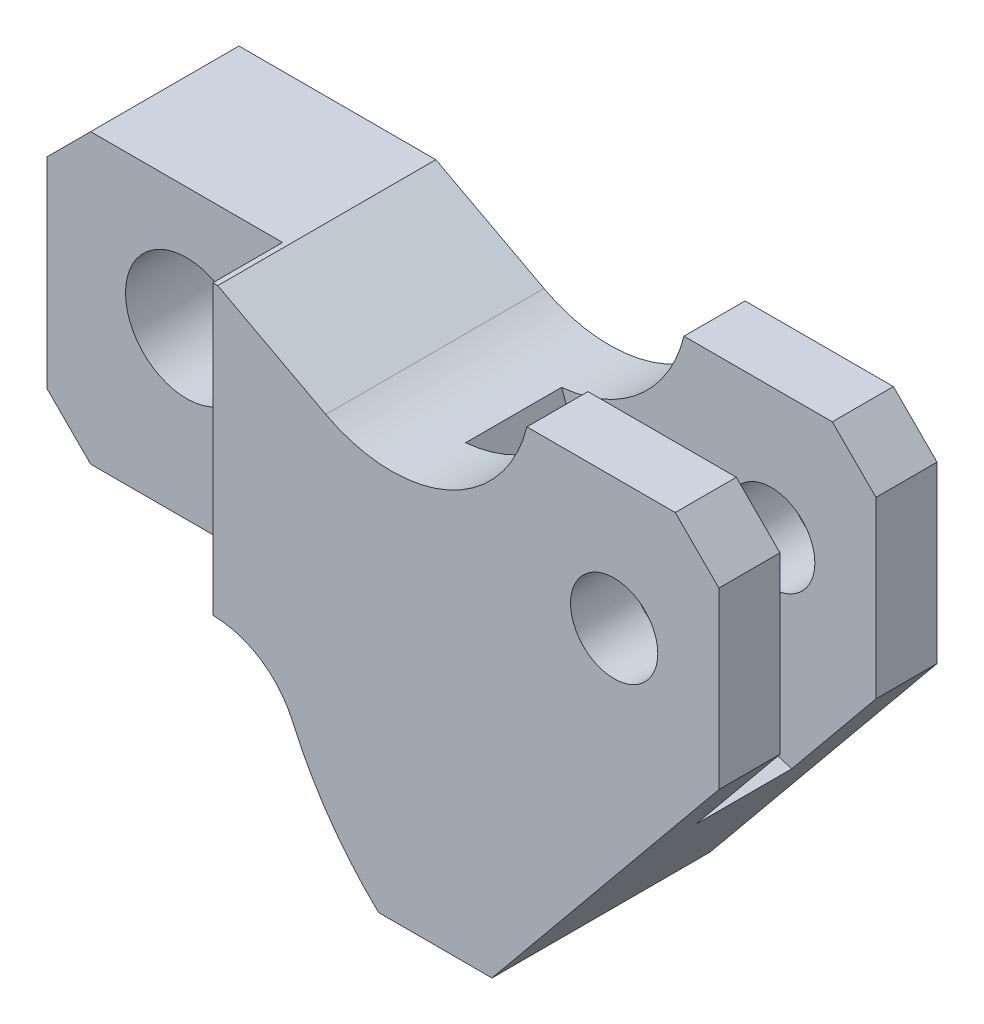
ISO-10303-21;
HEADER;
FILE_DESCRIPTION(('STEP AP214'),'2;1');
FILE_NAME('part.step','',(''),(''),'','','');
FILE_SCHEMA(('AUTOMOTIVE_DESIGN { 1 0 10303 214 1 1 1 1 }'));
ENDSEC;
DATA;
#1=APPLICATION_CONTEXT('core data for automotive mechanical design processes');
#2=APPLICATION_PROTOCOL_DEFINITION('international standard','automotive_design',2000,#1);
#3=PRODUCT_CONTEXT('',#1,'mechanical');
#4=PRODUCT('Part','Part','',(#3));
#5=PRODUCT_RELATED_PRODUCT_CATEGORY('part','',(#4));
#6=PRODUCT_DEFINITION_FORMATION('','',#4);
#7=PRODUCT_DEFINITION_CONTEXT('part definition',#1,'design');
#8=PRODUCT_DEFINITION('design','',#6,#7);
#9=PRODUCT_DEFINITION_SHAPE('','',#8);
#10=(LENGTH_UNIT() NAMED_UNIT(*) SI_UNIT(.MILLI.,.METRE.));
#11=(NAMED_UNIT(*) PLANE_ANGLE_UNIT() SI_UNIT($,.RADIAN.));
#12=(NAMED_UNIT(*) SI_UNIT($,.STERADIAN.) SOLID_ANGLE_UNIT());
#13=UNCERTAINTY_MEASURE_WITH_UNIT(LENGTH_MEASURE(1.E-05),#10,'distance_accuracy_value','');
#14=(GEOMETRIC_REPRESENTATION_CONTEXT(3) GLOBAL_UNCERTAINTY_ASSIGNED_CONTEXT((#13)) GLOBAL_UNIT_ASSIGNED_CONTEXT((#10,
#11,#12)) REPRESENTATION_CONTEXT('',''));
#15=CARTESIAN_POINT('',(0.,0.,0.));
#16=DIRECTION('',(0.,0.,1.));
#17=DIRECTION('',(1.,0.,0.));
#18=AXIS2_PLACEMENT_3D('',#15,#16,#17);
#19=CARTESIAN_POINT('',(11.5323662073749,-60.5393512020442,12.5));
#20=DIRECTION('',(-0.773189665661408,0.63417485042723,0.));
#21=DIRECTION('',(-0.63417485042723,-0.773189665661408,0.));
#22=AXIS2_PLACEMENT_3D('',#19,#20,#21);
#23=PLANE('',#22);
#24=DIRECTION('',(0.63417485042723,0.773189665661408,0.));
#25=VECTOR('',#24,1.);
#26=CARTESIAN_POINT('',(11.5323662073749,-60.5393512020442,-5.5));
#27=LINE('',#26,#25);
#28=CARTESIAN_POINT('',(27.8898245420085,-40.5962428742612,-5.5));
#29=VERTEX_POINT('',#28);
#30=CARTESIAN_POINT('',(37.5323662073748,-28.84,-5.5));
#31=VERTEX_POINT('',#30);
#32=EDGE_CURVE('E206',#29,#31,#27,.T.);
#33=ORIENTED_EDGE('',*,*,#32,.F.);
#34=DIRECTION('',(0.,0.,1.));
#35=VECTOR('',#34,1.);
#36=CARTESIAN_POINT('',(27.8898245420085,-40.5962428742612,-5.5));
#37=LINE('',#36,#35);
#38=CARTESIAN_POINT('',(27.8898245420085,-40.5962428742612,5.5));
#39=VERTEX_POINT('',#38);
#40=EDGE_CURVE('E200',#29,#39,#37,.T.);
#41=ORIENTED_EDGE('',*,*,#40,.T.);
#42=DIRECTION('',(0.63417485042723,0.773189665661408,0.));
#43=VECTOR('',#42,1.);
#44=CARTESIAN_POINT('',(11.5323662073749,-60.5393512020442,5.5));
#45=LINE('',#44,#43);
#46=CARTESIAN_POINT('',(37.5323662073748,-28.84,5.5));
#47=VERTEX_POINT('',#46);
#48=EDGE_CURVE('E186',#39,#47,#45,.T.);
#49=ORIENTED_EDGE('',*,*,#48,.T.);
#50=DIRECTION('',(0.,0.,-1.));
#51=VECTOR('',#50,1.);
#52=CARTESIAN_POINT('',(37.5323662073748,-28.84,12.5));
#53=LINE('',#52,#51);
#54=CARTESIAN_POINT('',(37.5323662073748,-28.84,12.5));
#55=VERTEX_POINT('',#54);
#56=EDGE_CURVE('E323',#55,#47,#53,.T.);
#57=ORIENTED_EDGE('',*,*,#56,.F.);
#58=DIRECTION('',(0.63417485042723,0.773189665661408,0.));
#59=VECTOR('',#58,1.);
#60=CARTESIAN_POINT('',(11.5323662073749,-60.5393512020442,12.5));
#61=LINE('',#60,#59);
#62=CARTESIAN_POINT('',(11.5323662073749,-60.5393512020442,12.5));
#63=VERTEX_POINT('',#62);
#64=EDGE_CURVE('E260',#63,#55,#61,.T.);
#65=ORIENTED_EDGE('',*,*,#64,.F.);
#66=DIRECTION('',(0.,0.,-1.));
#67=VECTOR('',#66,1.);
#68=CARTESIAN_POINT('',(11.5323662073749,-60.5393512020442,12.5));
#69=LINE('',#68,#67);
#70=CARTESIAN_POINT('',(11.5323662073749,-60.5393512020442,-12.5));
#71=VERTEX_POINT('',#70);
#72=EDGE_CURVE('E324',#63,#71,#69,.T.);
#73=ORIENTED_EDGE('',*,*,#72,.T.);
#74=DIRECTION('',(0.63417485042723,0.773189665661408,0.));
#75=VECTOR('',#74,1.);
#76=CARTESIAN_POINT('',(11.5323662073749,-60.5393512020442,-12.5));
#77=LINE('',#76,#75);
#78=CARTESIAN_POINT('',(37.5323662073748,-28.84,-12.5));
#79=VERTEX_POINT('',#78);
#80=EDGE_CURVE('E288',#71,#79,#77,.T.);
#81=ORIENTED_EDGE('',*,*,#80,.T.);
#82=EDGE_CURVE('E325',#31,#79,#53,.T.);
#83=ORIENTED_EDGE('',*,*,#82,.F.);
#84=EDGE_LOOP('',(#33,#41,#49,#57,#65,#73,#81,#83));
#85=FACE_BOUND('',#84,.T.);
#86=ADVANCED_FACE('F39',(#85),#23,.F.);
#87=CARTESIAN_POINT('',(37.5323662073748,-8.83999999999997,12.5));
#88=DIRECTION('',(-1.,0.,0.));
#89=DIRECTION('',(0.,-1.,0.));
#90=AXIS2_PLACEMENT_3D('',#87,#88,#89);
#91=PLANE('',#90);
#92=DIRECTION('',(0.,1.,0.));
#93=VECTOR('',#92,1.);
#94=CARTESIAN_POINT('',(37.5323662073748,-8.83999999999997,-5.5));
#95=LINE('',#94,#93);
#96=CARTESIAN_POINT('',(37.5323662073748,-8.83999999999997,-5.5));
#97=VERTEX_POINT('',#96);
#98=EDGE_CURVE('E209',#31,#97,#95,.T.);
#99=ORIENTED_EDGE('',*,*,#98,.F.);
#100=ORIENTED_EDGE('',*,*,#82,.T.);
#101=DIRECTION('',(0.,1.,0.));
#102=VECTOR('',#101,1.);
#103=CARTESIAN_POINT('',(37.5323662073748,-8.83999999999997,-12.5));
#104=LINE('',#103,#102);
#105=CARTESIAN_POINT('',(37.5323662073748,-8.83999999999997,-12.5));
#106=VERTEX_POINT('',#105);
#107=EDGE_CURVE('E291',#79,#106,#104,.T.);
#108=ORIENTED_EDGE('',*,*,#107,.T.);
#109=DIRECTION('',(0.,0.,-1.));
#110=VECTOR('',#109,1.);
#111=CARTESIAN_POINT('',(37.5323662073748,-8.83999999999997,12.5));
#112=LINE('',#111,#110);
#113=EDGE_CURVE('E318',#97,#106,#112,.T.);
#114=ORIENTED_EDGE('',*,*,#113,.F.);
#115=EDGE_LOOP('',(#99,#100,#108,#114));
#116=FACE_BOUND('',#115,.T.);
#117=ADVANCED_FACE('F375',(#116),#91,.F.);
#118=CARTESIAN_POINT('',(37.5323662073748,-8.83999999999997,12.5));
#119=DIRECTION('',(-0.707106781186546,-0.707106781186549,0.));
#120=DIRECTION('',(0.707106781186549,-0.707106781186546,0.));
#121=AXIS2_PLACEMENT_3D('',#118,#119,#120);
#122=PLANE('',#121);
#123=DIRECTION('',(-0.707106781186549,0.707106781186546,0.));
#124=VECTOR('',#123,1.);
#125=CARTESIAN_POINT('',(37.5323662073748,-8.83999999999997,-5.5));
#126=LINE('',#125,#124);
#127=CARTESIAN_POINT('',(32.5323662073748,-3.84,-5.5));
#128=VERTEX_POINT('',#127);
#129=EDGE_CURVE('E356',#97,#128,#126,.T.);
#130=ORIENTED_EDGE('',*,*,#129,.F.);
#131=ORIENTED_EDGE('',*,*,#113,.T.);
#132=DIRECTION('',(-0.707106781186549,0.707106781186546,0.));
#133=VECTOR('',#132,1.);
#134=CARTESIAN_POINT('',(37.5323662073748,-8.83999999999997,-12.5));
#135=LINE('',#134,#133);
#136=CARTESIAN_POINT('',(32.5323662073748,-3.84,-12.5));
#137=VERTEX_POINT('',#136);
#138=EDGE_CURVE('E296',#106,#137,#135,.T.);
#139=ORIENTED_EDGE('',*,*,#138,.T.);
#140=DIRECTION('',(0.,0.,-1.));
#141=VECTOR('',#140,1.);
#142=CARTESIAN_POINT('',(32.5323662073748,-3.84,12.5));
#143=LINE('',#142,#141);
#144=EDGE_CURVE('E314',#128,#137,#143,.T.);
#145=ORIENTED_EDGE('',*,*,#144,.F.);
#146=EDGE_LOOP('',(#130,#131,#139,#145));
#147=FACE_BOUND('',#146,.T.);
#148=ADVANCED_FACE('F371',(#147),#122,.F.);
#149=CARTESIAN_POINT('',(32.5323662073748,-3.84,12.5));
#150=DIRECTION('',(0.,-1.,0.));
#151=DIRECTION('',(1.,0.,0.));
#152=AXIS2_PLACEMENT_3D('',#149,#150,#151);
#153=PLANE('',#152);
#154=DIRECTION('',(-1.,0.,0.));
#155=VECTOR('',#154,1.);
#156=CARTESIAN_POINT('',(32.5323662073748,-3.84,-5.5));
#157=LINE('',#156,#155);
#158=CARTESIAN_POINT('',(15.5323662073748,-3.84,-5.5));
#159=VERTEX_POINT('',#158);
#160=EDGE_CURVE('E354',#128,#159,#157,.T.);
#161=ORIENTED_EDGE('',*,*,#160,.F.);
#162=ORIENTED_EDGE('',*,*,#144,.T.);
#163=DIRECTION('',(-1.,0.,0.));
#164=VECTOR('',#163,1.);
#165=CARTESIAN_POINT('',(32.5323662073748,-3.84,-12.5));
#166=LINE('',#165,#164);
#167=CARTESIAN_POINT('',(15.5323662073748,-3.84,-12.5));
#168=VERTEX_POINT('',#167);
#169=EDGE_CURVE('E298',#137,#168,#166,.T.);
#170=ORIENTED_EDGE('',*,*,#169,.T.);
#171=DIRECTION('',(0.,0.,-1.));
#172=VECTOR('',#171,1.);
#173=CARTESIAN_POINT('',(15.5323662073748,-3.84,12.5));
#174=LINE('',#173,#172);
#175=EDGE_CURVE('E309',#159,#168,#174,.T.);
#176=ORIENTED_EDGE('',*,*,#175,.F.);
#177=EDGE_LOOP('',(#161,#162,#170,#176));
#178=FACE_BOUND('',#177,.T.);
#179=ADVANCED_FACE('F384',(#178),#153,.F.);
#180=CARTESIAN_POINT('',(0.,0.,12.5));
#181=DIRECTION('',(0.,0.,-1.));
#182=DIRECTION('',(-1.,0.,0.));
#183=AXIS2_PLACEMENT_3D('',#180,#181,#182);
#184=CYLINDRICAL_SURFACE('',#183,16.);
#185=CARTESIAN_POINT('',(0.,0.,-5.5));
#186=DIRECTION('',(0.,0.,1.));
#187=DIRECTION('',(1.,0.,0.));
#188=AXIS2_PLACEMENT_3D('',#185,#186,#187);
#189=CIRCLE('',#188,16.);
#190=CARTESIAN_POINT('',(1.50656721275613,-15.9289125565259,-5.5));
#191=VERTEX_POINT('',#190);
#192=EDGE_CURVE('E355',#159,#191,#189,.F.);
#193=ORIENTED_EDGE('',*,*,#192,.F.);
#194=ORIENTED_EDGE('',*,*,#175,.T.);
#195=CARTESIAN_POINT('',(0.,0.,-12.5));
#196=DIRECTION('',(0.,0.,-1.));
#197=DIRECTION('',(1.,0.,0.));
#198=AXIS2_PLACEMENT_3D('',#195,#196,#197);
#199=CIRCLE('',#198,16.);
#200=CARTESIAN_POINT('',(-7.51154500457428,-14.1271614857428,-12.5));
#201=VERTEX_POINT('',#200);
#202=EDGE_CURVE('E304',#168,#201,#199,.T.);
#203=ORIENTED_EDGE('',*,*,#202,.T.);
#204=DIRECTION('',(0.,0.,-1.));
#205=VECTOR('',#204,1.);
#206=CARTESIAN_POINT('',(-7.51154500457428,-14.1271614857428,12.5));
#207=LINE('',#206,#205);
#208=CARTESIAN_POINT('',(-7.51154500457428,-14.1271614857428,12.5));
#209=VERTEX_POINT('',#208);
#210=EDGE_CURVE('E307',#209,#201,#207,.T.);
#211=ORIENTED_EDGE('',*,*,#210,.F.);
#212=CARTESIAN_POINT('',(0.,0.,12.5));
#213=DIRECTION('',(0.,0.,-1.));
#214=DIRECTION('',(1.,0.,0.));
#215=AXIS2_PLACEMENT_3D('',#212,#213,#214);
#216=CIRCLE('',#215,16.);
#217=CARTESIAN_POINT('',(15.5323662073748,-3.84,12.5));
#218=VERTEX_POINT('',#217);
#219=EDGE_CURVE('E264',#218,#209,#216,.T.);
#220=ORIENTED_EDGE('',*,*,#219,.F.);
#221=CARTESIAN_POINT('',(15.5323662073748,-3.84,5.5));
#222=VERTEX_POINT('',#221);
#223=EDGE_CURVE('E313',#218,#222,#174,.T.);
#224=ORIENTED_EDGE('',*,*,#223,.T.);
#225=CARTESIAN_POINT('',(0.,0.,5.5));
#226=DIRECTION('',(0.,0.,1.));
#227=DIRECTION('',(1.,0.,0.));
#228=AXIS2_PLACEMENT_3D('',#225,#226,#227);
#229=CIRCLE('',#228,16.);
#230=CARTESIAN_POINT('',(1.50656721275613,-15.9289125565259,5.5));
#231=VERTEX_POINT('',#230);
#232=EDGE_CURVE('E348',#222,#231,#229,.F.);
#233=ORIENTED_EDGE('',*,*,#232,.T.);
#234=DIRECTION('',(0.,0.,1.));
#235=VECTOR('',#234,1.);
#236=CARTESIAN_POINT('',(1.50656721275613,-15.9289125565259,0.));
#237=LINE('',#236,#235);
#238=EDGE_CURVE('E11',#231,#191,#237,.F.);
#239=ORIENTED_EDGE('',*,*,#238,.T.);
#240=EDGE_LOOP('',(#193,#194,#203,#211,#220,#224,#233,#239));
#241=FACE_BOUND('',#240,.T.);
#242=ADVANCED_FACE('F390',(#241),#184,.F.);
#243=CARTESIAN_POINT('',(25.5323662073748,-18.84,12.5));
#244=DIRECTION('',(0.,0.,-1.));
#245=DIRECTION('',(-1.,0.,0.));
#246=AXIS2_PLACEMENT_3D('',#243,#244,#245);
#247=CYLINDRICAL_SURFACE('',#246,5.);
#248=CARTESIAN_POINT('',(25.5323662073748,-18.84,-12.5));
#249=DIRECTION('',(0.,0.,1.));
#250=DIRECTION('',(1.,0.,0.));
#251=AXIS2_PLACEMENT_3D('',#248,#249,#250);
#252=CIRCLE('',#251,5.);
#253=CARTESIAN_POINT('',(30.5323662073748,-18.84,-12.5));
#254=VERTEX_POINT('',#253);
#255=EDGE_CURVE('E238',#254,#254,#252,.T.);
#256=ORIENTED_EDGE('',*,*,#255,.F.);
#257=EDGE_LOOP('',(#256));
#258=FACE_BOUND('',#257,.T.);
#259=CARTESIAN_POINT('',(25.5323662073748,-18.84,-5.5));
#260=DIRECTION('',(0.,0.,1.));
#261=DIRECTION('',(1.,0.,0.));
#262=AXIS2_PLACEMENT_3D('',#259,#260,#261);
#263=CIRCLE('',#262,5.);
#264=CARTESIAN_POINT('',(30.5323662073748,-18.84,-5.5));
#265=VERTEX_POINT('',#264);
#266=EDGE_CURVE('E191',#265,#265,#263,.T.);
#267=ORIENTED_EDGE('',*,*,#266,.T.);
#268=EDGE_LOOP('',(#267));
#269=FACE_BOUND('',#268,.T.);
#270=ADVANCED_FACE('F521',(#258,#269),#247,.F.);
#271=CARTESIAN_POINT('',(0.,0.,12.5));
#272=DIRECTION('',(0.,0.,1.));
#273=DIRECTION('',(1.,0.,0.));
#274=AXIS2_PLACEMENT_3D('',#271,#272,#273);
#275=PLANE('',#274);
#276=DIRECTION('',(0.,1.,0.));
#277=VECTOR('',#276,1.);
#278=CARTESIAN_POINT('',(-20.4676337926252,-63.,12.5));
#279=LINE('',#278,#277);
#280=CARTESIAN_POINT('',(-20.4676337926252,-40.5393512047768,12.5));
#281=VERTEX_POINT('',#280);
#282=CARTESIAN_POINT('',(-20.4676337926252,-7.53935120204417,12.5));
#283=VERTEX_POINT('',#282);
#284=EDGE_CURVE('E210',#281,#283,#279,.T.);
#285=ORIENTED_EDGE('',*,*,#284,.F.);
#286=CARTESIAN_POINT('',(-20.4678675737837,-50.5393512020442,12.5));
#287=DIRECTION('',(0.,0.,-1.));
#288=DIRECTION('',(1.,0.,0.));
#289=AXIS2_PLACEMENT_3D('',#286,#287,#288);
#290=CIRCLE('',#289,10.);
#291=CARTESIAN_POINT('',(-11.3046871064585,-46.5348382824457,12.5));
#292=VERTEX_POINT('',#291);
#293=EDGE_CURVE('E248',#281,#292,#290,.T.);
#294=ORIENTED_EDGE('',*,*,#293,.T.);
#295=CARTESIAN_POINT('',(28.0969889030397,-29.3154327281725,12.5));
#296=DIRECTION('',(0.,0.,1.));
#297=DIRECTION('',(-1.,0.,0.));
#298=AXIS2_PLACEMENT_3D('',#295,#296,#297);
#299=CIRCLE('',#298,43.);
#300=CARTESIAN_POINT('',(-1.46763379262514,-60.5393512020442,12.5));
#301=VERTEX_POINT('',#300);
#302=EDGE_CURVE('E251',#292,#301,#299,.T.);
#303=ORIENTED_EDGE('',*,*,#302,.T.);
#304=DIRECTION('',(1.,0.,0.));
#305=VECTOR('',#304,1.);
#306=CARTESIAN_POINT('',(-1.46763379262515,-60.5393512020442,12.5));
#307=LINE('',#306,#305);
#308=EDGE_CURVE('E254',#301,#63,#307,.T.);
#309=ORIENTED_EDGE('',*,*,#308,.T.);
#310=ORIENTED_EDGE('',*,*,#64,.T.);
#311=DIRECTION('',(0.,1.,0.));
#312=VECTOR('',#311,1.);
#313=CARTESIAN_POINT('',(37.5323662073748,-8.83999999999997,12.5));
#314=LINE('',#313,#312);
#315=CARTESIAN_POINT('',(37.5323662073748,-8.83999999999997,12.5));
#316=VERTEX_POINT('',#315);
#317=EDGE_CURVE('E259',#55,#316,#314,.T.);
#318=ORIENTED_EDGE('',*,*,#317,.T.);
#319=DIRECTION('',(-0.707106781186549,0.707106781186546,0.));
#320=VECTOR('',#319,1.);
#321=CARTESIAN_POINT('',(37.5323662073748,-8.83999999999997,12.5));
#322=LINE('',#321,#320);
#323=CARTESIAN_POINT('',(32.5323662073748,-3.84,12.5));
#324=VERTEX_POINT('',#323);
#325=EDGE_CURVE('E261',#316,#324,#322,.T.);
#326=ORIENTED_EDGE('',*,*,#325,.T.);
#327=DIRECTION('',(-1.,0.,0.));
#328=VECTOR('',#327,1.);
#329=CARTESIAN_POINT('',(32.5323662073748,-3.84,12.5));
#330=LINE('',#329,#328);
#331=EDGE_CURVE('E263',#324,#218,#330,.T.);
#332=ORIENTED_EDGE('',*,*,#331,.T.);
#333=ORIENTED_EDGE('',*,*,#219,.T.);
#334=DIRECTION('',(-0.882947592858926,0.469471562785892,0.));
#335=VECTOR('',#334,1.);
#336=CARTESIAN_POINT('',(-19.901414153807,-7.53935120204417,12.5));
#337=LINE('',#336,#335);
#338=CARTESIAN_POINT('',(-19.901414153807,-7.53935120204417,12.5));
#339=VERTEX_POINT('',#338);
#340=EDGE_CURVE('E270',#209,#339,#337,.T.);
#341=ORIENTED_EDGE('',*,*,#340,.T.);
#342=DIRECTION('',(-1.,0.,0.));
#343=VECTOR('',#342,1.);
#344=CARTESIAN_POINT('',(-42.4676337926252,-7.53935120204417,12.5));
#345=LINE('',#344,#343);
#346=EDGE_CURVE('E249',#339,#283,#345,.T.);
#347=ORIENTED_EDGE('',*,*,#346,.T.);
#348=EDGE_LOOP('',(#285,#294,#303,#309,#310,#318,#326,#332,#333,#341,#347));
#349=FACE_BOUND('',#348,.T.);
#350=CARTESIAN_POINT('',(25.5323662073748,-18.84,12.5));
#351=DIRECTION('',(0.,0.,1.));
#352=DIRECTION('',(1.,0.,0.));
#353=AXIS2_PLACEMENT_3D('',#350,#351,#352);
#354=CIRCLE('',#353,5.);
#355=CARTESIAN_POINT('',(30.5323662073748,-18.84,12.5));
#356=VERTEX_POINT('',#355);
#357=EDGE_CURVE('E241',#356,#356,#354,.T.);
#358=ORIENTED_EDGE('',*,*,#357,.F.);
#359=EDGE_LOOP('',(#358));
#360=FACE_BOUND('',#359,.T.);
#361=ADVANCED_FACE('F408',(#349,#360),#275,.T.);
#362=CARTESIAN_POINT('',(0.,0.,-12.5));
#363=DIRECTION('',(0.,0.,1.));
#364=DIRECTION('',(1.,0.,0.));
#365=AXIS2_PLACEMENT_3D('',#362,#363,#364);
#366=PLANE('',#365);
#367=DIRECTION('',(-1.,0.,0.));
#368=VECTOR('',#367,1.);
#369=CARTESIAN_POINT('',(-42.4676337926252,-7.53935120204417,-12.5));
#370=LINE('',#369,#368);
#371=CARTESIAN_POINT('',(-19.901414153807,-7.53935120204417,-12.5));
#372=VERTEX_POINT('',#371);
#373=CARTESIAN_POINT('',(-42.4676337926252,-7.53935120204417,-12.5));
#374=VERTEX_POINT('',#373);
#375=EDGE_CURVE('E243',#372,#374,#370,.T.);
#376=ORIENTED_EDGE('',*,*,#375,.F.);
#377=DIRECTION('',(-0.882947592858926,0.469471562785892,0.));
#378=VECTOR('',#377,1.);
#379=CARTESIAN_POINT('',(-19.901414153807,-7.53935120204417,-12.5));
#380=LINE('',#379,#378);
#381=EDGE_CURVE('E253',#201,#372,#380,.T.);
#382=ORIENTED_EDGE('',*,*,#381,.F.);
#383=ORIENTED_EDGE('',*,*,#202,.F.);
#384=ORIENTED_EDGE('',*,*,#169,.F.);
#385=ORIENTED_EDGE('',*,*,#138,.F.);
#386=ORIENTED_EDGE('',*,*,#107,.F.);
#387=ORIENTED_EDGE('',*,*,#80,.F.);
#388=DIRECTION('',(1.,0.,0.));
#389=VECTOR('',#388,1.);
#390=CARTESIAN_POINT('',(-1.46763379262515,-60.5393512020442,-12.5));
#391=LINE('',#390,#389);
#392=CARTESIAN_POINT('',(-1.46763379262514,-60.5393512020442,-12.5));
#393=VERTEX_POINT('',#392);
#394=EDGE_CURVE('E290',#393,#71,#391,.T.);
#395=ORIENTED_EDGE('',*,*,#394,.F.);
#396=CARTESIAN_POINT('',(28.0969889030397,-29.3154327281725,-12.5));
#397=DIRECTION('',(0.,0.,1.));
#398=DIRECTION('',(-1.,0.,0.));
#399=AXIS2_PLACEMENT_3D('',#396,#397,#398);
#400=CIRCLE('',#399,43.);
#401=CARTESIAN_POINT('',(-11.3046871064585,-46.5348382824457,-12.5));
#402=VERTEX_POINT('',#401);
#403=EDGE_CURVE('E287',#402,#393,#400,.T.);
#404=ORIENTED_EDGE('',*,*,#403,.F.);
#405=CARTESIAN_POINT('',(-20.4678675737837,-50.5393512020442,-12.5));
#406=DIRECTION('',(0.,0.,-1.));
#407=DIRECTION('',(1.,0.,0.));
#408=AXIS2_PLACEMENT_3D('',#405,#406,#407);
#409=CIRCLE('',#408,10.);
#410=CARTESIAN_POINT('',(-20.4678675737837,-40.5393512020442,-12.5));
#411=VERTEX_POINT('',#410);
#412=EDGE_CURVE('E283',#411,#402,#409,.T.);
#413=ORIENTED_EDGE('',*,*,#412,.F.);
#414=DIRECTION('',(1.,0.,0.));
#415=VECTOR('',#414,1.);
#416=CARTESIAN_POINT('',(-42.4676337926252,-40.5393512020442,-12.5));
#417=LINE('',#416,#415);
#418=CARTESIAN_POINT('',(-42.4676337926252,-40.5393512020442,-12.5));
#419=VERTEX_POINT('',#418);
#420=EDGE_CURVE('E281',#419,#411,#417,.T.);
#421=ORIENTED_EDGE('',*,*,#420,.F.);
#422=DIRECTION('',(0.707106781186547,-0.707106781186549,0.));
#423=VECTOR('',#422,1.);
#424=CARTESIAN_POINT('',(-47.4676337926252,-35.5393512020442,-12.5));
#425=LINE('',#424,#423);
#426=CARTESIAN_POINT('',(-47.4676337926252,-35.5393512020442,-12.5));
#427=VERTEX_POINT('',#426);
#428=EDGE_CURVE('E279',#427,#419,#425,.T.);
#429=ORIENTED_EDGE('',*,*,#428,.F.);
#430=DIRECTION('',(0.,-1.,0.));
#431=VECTOR('',#430,1.);
#432=CARTESIAN_POINT('',(-47.4676337926252,-12.5393512020442,-12.5));
#433=LINE('',#432,#431);
#434=CARTESIAN_POINT('',(-47.4676337926252,-12.5393512020442,-12.5));
#435=VERTEX_POINT('',#434);
#436=EDGE_CURVE('E274',#435,#427,#433,.T.);
#437=ORIENTED_EDGE('',*,*,#436,.F.);
#438=DIRECTION('',(-0.707106781186549,-0.707106781186547,0.));
#439=VECTOR('',#438,1.);
#440=CARTESIAN_POINT('',(-47.4676337926252,-12.5393512020442,-12.5));
#441=LINE('',#440,#439);
#442=EDGE_CURVE('E275',#374,#435,#441,.T.);
#443=ORIENTED_EDGE('',*,*,#442,.F.);
#444=EDGE_LOOP('',(#376,#382,#383,#384,#385,#386,#387,#395,#404,#413,#421,#429,#437,#443));
#445=FACE_BOUND('',#444,.T.);
#446=ORIENTED_EDGE('',*,*,#255,.T.);
#447=EDGE_LOOP('',(#446));
#448=FACE_BOUND('',#447,.T.);
#449=CARTESIAN_POINT('',(-31.4676337926252,-21.5393512020442,-12.5));
#450=DIRECTION('',(0.,0.,1.));
#451=DIRECTION('',(1.,0.,0.));
#452=AXIS2_PLACEMENT_3D('',#449,#450,#451);
#453=CIRCLE('',#452,7.);
#454=CARTESIAN_POINT('',(-24.4676337926252,-21.5393512020442,-12.5));
#455=VERTEX_POINT('',#454);
#456=EDGE_CURVE('E240',#455,#455,#453,.T.);
#457=ORIENTED_EDGE('',*,*,#456,.T.);
#458=EDGE_LOOP('',(#457));
#459=FACE_BOUND('',#458,.T.);
#460=ADVANCED_FACE('F377',(#445,#448,#459),#366,.F.);
#461=CARTESIAN_POINT('',(-42.4676337926252,-7.53935120204417,12.5));
#462=DIRECTION('',(0.,-1.,0.));
#463=DIRECTION('',(0.,0.,-1.));
#464=AXIS2_PLACEMENT_3D('',#461,#462,#463);
#465=PLANE('',#464);
#466=DIRECTION('',(0.,0.,-1.));
#467=VECTOR('',#466,1.);
#468=CARTESIAN_POINT('',(-42.4676337926252,-7.53935120204417,12.5));
#469=LINE('',#468,#467);
#470=CARTESIAN_POINT('',(-42.4676337926252,-7.53935120204417,4.5));
#471=VERTEX_POINT('',#470);
#472=EDGE_CURVE('E344',#471,#374,#469,.T.);
#473=ORIENTED_EDGE('',*,*,#472,.F.);
#474=DIRECTION('',(1.,0.,0.));
#475=VECTOR('',#474,1.);
#476=CARTESIAN_POINT('',(-42.4676337926252,-7.53935120204417,4.5));
#477=LINE('',#476,#475);
#478=CARTESIAN_POINT('',(-20.4676337926252,-7.53935120204417,4.5));
#479=VERTEX_POINT('',#478);
#480=EDGE_CURVE('E232',#471,#479,#477,.T.);
#481=ORIENTED_EDGE('',*,*,#480,.T.);
#482=DIRECTION('',(0.,0.,1.));
#483=VECTOR('',#482,1.);
#484=CARTESIAN_POINT('',(-20.4676337926252,-7.53935120204417,12.5));
#485=LINE('',#484,#483);
#486=EDGE_CURVE('E231',#479,#283,#485,.T.);
#487=ORIENTED_EDGE('',*,*,#486,.T.);
#488=ORIENTED_EDGE('',*,*,#346,.F.);
#489=DIRECTION('',(0.,0.,-1.));
#490=VECTOR('',#489,1.);
#491=CARTESIAN_POINT('',(-19.901414153807,-7.53935120204417,12.5));
#492=LINE('',#491,#490);
#493=EDGE_CURVE('E267',#339,#372,#492,.T.);
#494=ORIENTED_EDGE('',*,*,#493,.T.);
#495=ORIENTED_EDGE('',*,*,#375,.T.);
#496=EDGE_LOOP('',(#473,#481,#487,#488,#494,#495));
#497=FACE_BOUND('',#496,.T.);
#498=ADVANCED_FACE('F41',(#497),#465,.F.);
#499=CARTESIAN_POINT('',(-47.4676337926252,-12.5393512020442,12.5));
#500=DIRECTION('',(0.707106781186547,-0.707106781186548,0.));
#501=DIRECTION('',(0.707106781186548,0.707106781186547,0.));
#502=AXIS2_PLACEMENT_3D('',#499,#500,#501);
#503=PLANE('',#502);
#504=DIRECTION('',(0.,0.,-1.));
#505=VECTOR('',#504,1.);
#506=CARTESIAN_POINT('',(-47.4676337926252,-12.5393512020442,12.5));
#507=LINE('',#506,#505);
#508=CARTESIAN_POINT('',(-47.4676337926252,-12.5393512020441,4.5));
#509=VERTEX_POINT('',#508);
#510=EDGE_CURVE('E339',#509,#435,#507,.T.);
#511=ORIENTED_EDGE('',*,*,#510,.F.);
#512=DIRECTION('',(0.707106781186548,0.707106781186547,0.));
#513=VECTOR('',#512,1.);
#514=CARTESIAN_POINT('',(-47.4676337926252,-12.5393512020442,4.5));
#515=LINE('',#514,#513);
#516=EDGE_CURVE('E227',#509,#471,#515,.T.);
#517=ORIENTED_EDGE('',*,*,#516,.T.);
#518=ORIENTED_EDGE('',*,*,#472,.T.);
#519=ORIENTED_EDGE('',*,*,#442,.T.);
#520=EDGE_LOOP('',(#511,#517,#518,#519));
#521=FACE_BOUND('',#520,.T.);
#522=ADVANCED_FACE('F455',(#521),#503,.F.);
#523=CARTESIAN_POINT('',(-47.4676337926252,-12.5393512020442,12.5));
#524=DIRECTION('',(1.,0.,0.));
#525=DIRECTION('',(0.,0.,-1.));
#526=AXIS2_PLACEMENT_3D('',#523,#524,#525);
#527=PLANE('',#526);
#528=DIRECTION('',(0.,0.,-1.));
#529=VECTOR('',#528,1.);
#530=CARTESIAN_POINT('',(-47.4676337926252,-35.5393512020442,12.5));
#531=LINE('',#530,#529);
#532=CARTESIAN_POINT('',(-47.4676337926252,-35.5393512020442,4.5));
#533=VERTEX_POINT('',#532);
#534=EDGE_CURVE('E337',#533,#427,#531,.T.);
#535=ORIENTED_EDGE('',*,*,#534,.F.);
#536=DIRECTION('',(0.,1.,0.));
#537=VECTOR('',#536,1.);
#538=CARTESIAN_POINT('',(-47.4676337926252,-63.,4.5));
#539=LINE('',#538,#537);
#540=EDGE_CURVE('E212',#533,#509,#539,.T.);
#541=ORIENTED_EDGE('',*,*,#540,.T.);
#542=ORIENTED_EDGE('',*,*,#510,.T.);
#543=ORIENTED_EDGE('',*,*,#436,.T.);
#544=EDGE_LOOP('',(#535,#541,#542,#543));
#545=FACE_BOUND('',#544,.T.);
#546=ADVANCED_FACE('F437',(#545),#527,.F.);
#547=CARTESIAN_POINT('',(-47.4676337926252,-35.5393512020442,12.5));
#548=DIRECTION('',(0.707106781186548,0.707106781186547,0.));
#549=DIRECTION('',(-0.707106781186547,0.707106781186548,0.));
#550=AXIS2_PLACEMENT_3D('',#547,#548,#549);
#551=PLANE('',#550);
#552=DIRECTION('',(0.,0.,-1.));
#553=VECTOR('',#552,1.);
#554=CARTESIAN_POINT('',(-42.4676337926252,-40.5393512020442,12.5));
#555=LINE('',#554,#553);
#556=CARTESIAN_POINT('',(-42.4676337926252,-40.5393512020442,4.5));
#557=VERTEX_POINT('',#556);
#558=EDGE_CURVE('E336',#557,#419,#555,.T.);
#559=ORIENTED_EDGE('',*,*,#558,.F.);
#560=DIRECTION('',(-0.707106781186547,0.707106781186548,0.));
#561=VECTOR('',#560,1.);
#562=CARTESIAN_POINT('',(-47.4676337926252,-35.5393512020442,4.5));
#563=LINE('',#562,#561);
#564=EDGE_CURVE('E223',#557,#533,#563,.T.);
#565=ORIENTED_EDGE('',*,*,#564,.T.);
#566=ORIENTED_EDGE('',*,*,#534,.T.);
#567=ORIENTED_EDGE('',*,*,#428,.T.);
#568=EDGE_LOOP('',(#559,#565,#566,#567));
#569=FACE_BOUND('',#568,.T.);
#570=ADVANCED_FACE('F434',(#569),#551,.F.);
#571=CARTESIAN_POINT('',(-42.4676337926252,-40.5393512020442,12.5));
#572=DIRECTION('',(0.,1.,0.));
#573=DIRECTION('',(0.,0.,1.));
#574=AXIS2_PLACEMENT_3D('',#571,#572,#573);
#575=PLANE('',#574);
#576=DIRECTION('',(0.,0.,-1.));
#577=VECTOR('',#576,1.);
#578=CARTESIAN_POINT('',(-20.4678675737837,-40.5393512020442,12.5));
#579=LINE('',#578,#577);
#580=CARTESIAN_POINT('',(-20.4678675737837,-40.5393512020442,4.5));
#581=VERTEX_POINT('',#580);
#582=EDGE_CURVE('E331',#581,#411,#579,.T.);
#583=ORIENTED_EDGE('',*,*,#582,.F.);
#584=DIRECTION('',(-1.,0.,0.));
#585=VECTOR('',#584,1.);
#586=CARTESIAN_POINT('',(-42.4676337926252,-40.5393512020442,4.5));
#587=LINE('',#586,#585);
#588=EDGE_CURVE('E225',#581,#557,#587,.T.);
#589=ORIENTED_EDGE('',*,*,#588,.T.);
#590=ORIENTED_EDGE('',*,*,#558,.T.);
#591=ORIENTED_EDGE('',*,*,#420,.T.);
#592=EDGE_LOOP('',(#583,#589,#590,#591));
#593=FACE_BOUND('',#592,.T.);
#594=ADVANCED_FACE('F435',(#593),#575,.F.);
#595=CARTESIAN_POINT('',(-20.4678675737837,-50.5393512020442,12.5));
#596=DIRECTION('',(0.,0.,-1.));
#597=DIRECTION('',(-1.,0.,0.));
#598=AXIS2_PLACEMENT_3D('',#595,#596,#597);
#599=CYLINDRICAL_SURFACE('',#598,10.);
#600=DIRECTION('',(0.,0.,-1.));
#601=VECTOR('',#600,1.);
#602=CARTESIAN_POINT('',(-20.4676337926252,-40.5393512047768,12.5));
#603=LINE('',#602,#601);
#604=CARTESIAN_POINT('',(-20.4676337926252,-40.5393512047768,4.5));
#605=VERTEX_POINT('',#604);
#606=EDGE_CURVE('E50',#281,#605,#603,.T.);
#607=ORIENTED_EDGE('',*,*,#606,.T.);
#608=CARTESIAN_POINT('',(-20.4678675737837,-50.5393512020442,4.5));
#609=DIRECTION('',(0.,0.,-1.));
#610=DIRECTION('',(-1.,0.,0.));
#611=AXIS2_PLACEMENT_3D('',#608,#609,#610);
#612=CIRCLE('',#611,10.);
#613=EDGE_CURVE('E218',#605,#581,#612,.F.);
#614=ORIENTED_EDGE('',*,*,#613,.T.);
#615=ORIENTED_EDGE('',*,*,#582,.T.);
#616=ORIENTED_EDGE('',*,*,#412,.T.);
#617=DIRECTION('',(0.,0.,-1.));
#618=VECTOR('',#617,1.);
#619=CARTESIAN_POINT('',(-11.3046871064585,-46.5348382824457,12.5));
#620=LINE('',#619,#618);
#621=EDGE_CURVE('E332',#292,#402,#620,.T.);
#622=ORIENTED_EDGE('',*,*,#621,.F.);
#623=ORIENTED_EDGE('',*,*,#293,.F.);
#624=EDGE_LOOP('',(#607,#614,#615,#616,#622,#623));
#625=FACE_BOUND('',#624,.T.);
#626=ADVANCED_FACE('F426',(#625),#599,.F.);
#627=CARTESIAN_POINT('',(28.0969889030397,-29.3154327281725,12.5));
#628=DIRECTION('',(0.,0.,-1.));
#629=DIRECTION('',(-1.,0.,0.));
#630=AXIS2_PLACEMENT_3D('',#627,#628,#629);
#631=CYLINDRICAL_SURFACE('',#630,43.);
#632=ORIENTED_EDGE('',*,*,#403,.T.);
#633=DIRECTION('',(0.,0.,-1.));
#634=VECTOR('',#633,1.);
#635=CARTESIAN_POINT('',(-1.46763379262514,-60.5393512020442,12.5));
#636=LINE('',#635,#634);
#637=EDGE_CURVE('E327',#301,#393,#636,.T.);
#638=ORIENTED_EDGE('',*,*,#637,.F.);
#639=ORIENTED_EDGE('',*,*,#302,.F.);
#640=ORIENTED_EDGE('',*,*,#621,.T.);
#641=EDGE_LOOP('',(#632,#638,#639,#640));
#642=FACE_BOUND('',#641,.T.);
#643=ADVANCED_FACE('F425',(#642),#631,.T.);
#644=CARTESIAN_POINT('',(-1.46763379262515,-60.5393512020442,12.5));
#645=DIRECTION('',(0.,1.,0.));
#646=DIRECTION('',(0.,0.,1.));
#647=AXIS2_PLACEMENT_3D('',#644,#645,#646);
#648=PLANE('',#647);
#649=ORIENTED_EDGE('',*,*,#394,.T.);
#650=ORIENTED_EDGE('',*,*,#72,.F.);
#651=ORIENTED_EDGE('',*,*,#308,.F.);
#652=ORIENTED_EDGE('',*,*,#637,.T.);
#653=EDGE_LOOP('',(#649,#650,#651,#652));
#654=FACE_BOUND('',#653,.T.);
#655=ADVANCED_FACE('F416',(#654),#648,.F.);
#656=ORIENTED_EDGE('',*,*,#56,.T.);
#657=DIRECTION('',(0.,1.,0.));
#658=VECTOR('',#657,1.);
#659=CARTESIAN_POINT('',(37.5323662073748,-8.83999999999997,5.5));
#660=LINE('',#659,#658);
#661=CARTESIAN_POINT('',(37.5323662073748,-8.83999999999997,5.5));
#662=VERTEX_POINT('',#661);
#663=EDGE_CURVE('E188',#47,#662,#660,.T.);
#664=ORIENTED_EDGE('',*,*,#663,.T.);
#665=EDGE_CURVE('E317',#316,#662,#112,.T.);
#666=ORIENTED_EDGE('',*,*,#665,.F.);
#667=ORIENTED_EDGE('',*,*,#317,.F.);
#668=EDGE_LOOP('',(#656,#664,#666,#667));
#669=FACE_BOUND('',#668,.T.);
#670=ADVANCED_FACE('F398',(#669),#91,.F.);
#671=ORIENTED_EDGE('',*,*,#665,.T.);
#672=DIRECTION('',(-0.707106781186549,0.707106781186546,0.));
#673=VECTOR('',#672,1.);
#674=CARTESIAN_POINT('',(37.5323662073748,-8.83999999999997,5.5));
#675=LINE('',#674,#673);
#676=CARTESIAN_POINT('',(32.5323662073748,-3.84,5.5));
#677=VERTEX_POINT('',#676);
#678=EDGE_CURVE('E392',#662,#677,#675,.T.);
#679=ORIENTED_EDGE('',*,*,#678,.T.);
#680=EDGE_CURVE('E312',#324,#677,#143,.T.);
#681=ORIENTED_EDGE('',*,*,#680,.F.);
#682=ORIENTED_EDGE('',*,*,#325,.F.);
#683=EDGE_LOOP('',(#671,#679,#681,#682));
#684=FACE_BOUND('',#683,.T.);
#685=ADVANCED_FACE('F404',(#684),#122,.F.);
#686=ORIENTED_EDGE('',*,*,#680,.T.);
#687=DIRECTION('',(-1.,0.,0.));
#688=VECTOR('',#687,1.);
#689=CARTESIAN_POINT('',(32.5323662073748,-3.84,5.5));
#690=LINE('',#689,#688);
#691=EDGE_CURVE('E391',#677,#222,#690,.T.);
#692=ORIENTED_EDGE('',*,*,#691,.T.);
#693=ORIENTED_EDGE('',*,*,#223,.F.);
#694=ORIENTED_EDGE('',*,*,#331,.F.);
#695=EDGE_LOOP('',(#686,#692,#693,#694));
#696=FACE_BOUND('',#695,.T.);
#697=ADVANCED_FACE('F550',(#696),#153,.F.);
#698=CARTESIAN_POINT('',(-19.901414153807,-7.53935120204417,12.5));
#699=DIRECTION('',(-0.469471562785892,-0.882947592858926,0.));
#700=DIRECTION('',(0.882947592858926,-0.469471562785892,0.));
#701=AXIS2_PLACEMENT_3D('',#698,#699,#700);
#702=PLANE('',#701);
#703=ORIENTED_EDGE('',*,*,#381,.T.);
#704=ORIENTED_EDGE('',*,*,#493,.F.);
#705=ORIENTED_EDGE('',*,*,#340,.F.);
#706=ORIENTED_EDGE('',*,*,#210,.T.);
#707=EDGE_LOOP('',(#703,#704,#705,#706));
#708=FACE_BOUND('',#707,.T.);
#709=ADVANCED_FACE('F447',(#708),#702,.F.);
#710=CARTESIAN_POINT('',(25.5323662073748,-18.84,5.5));
#711=DIRECTION('',(0.,0.,1.));
#712=DIRECTION('',(1.,0.,0.));
#713=AXIS2_PLACEMENT_3D('',#710,#711,#712);
#714=CIRCLE('',#713,5.);
#715=CARTESIAN_POINT('',(30.5323662073748,-18.84,5.5));
#716=VERTEX_POINT('',#715);
#717=EDGE_CURVE('E346',#716,#716,#714,.T.);
#718=ORIENTED_EDGE('',*,*,#717,.F.);
#719=EDGE_LOOP('',(#718));
#720=FACE_BOUND('',#719,.T.);
#721=ORIENTED_EDGE('',*,*,#357,.T.);
#722=EDGE_LOOP('',(#721));
#723=FACE_BOUND('',#722,.T.);
#724=ADVANCED_FACE('F501',(#720,#723),#247,.F.);
#725=CARTESIAN_POINT('',(-31.4676337926252,-21.5393512020442,12.5));
#726=DIRECTION('',(0.,0.,-1.));
#727=DIRECTION('',(-1.,0.,0.));
#728=AXIS2_PLACEMENT_3D('',#725,#726,#727);
#729=CYLINDRICAL_SURFACE('',#728,7.);
#730=CARTESIAN_POINT('',(-31.4676337926252,-21.5393512020442,4.5));
#731=DIRECTION('',(0.,0.,-1.));
#732=DIRECTION('',(-1.,0.,0.));
#733=AXIS2_PLACEMENT_3D('',#730,#731,#732);
#734=CIRCLE('',#733,7.);
#735=CARTESIAN_POINT('',(-38.4676337926252,-21.5393512020442,4.5));
#736=VERTEX_POINT('',#735);
#737=EDGE_CURVE('E220',#736,#736,#734,.T.);
#738=ORIENTED_EDGE('',*,*,#737,.F.);
#739=EDGE_LOOP('',(#738));
#740=FACE_BOUND('',#739,.T.);
#741=ORIENTED_EDGE('',*,*,#456,.F.);
#742=EDGE_LOOP('',(#741));
#743=FACE_BOUND('',#742,.T.);
#744=ADVANCED_FACE('F500',(#740,#743),#729,.F.);
#745=CARTESIAN_POINT('',(-20.4676337926252,-63.,12.5));
#746=DIRECTION('',(1.,0.,0.));
#747=DIRECTION('',(0.,0.,-1.));
#748=AXIS2_PLACEMENT_3D('',#745,#746,#747);
#749=PLANE('',#748);
#750=DIRECTION('',(0.,1.,0.));
#751=VECTOR('',#750,1.);
#752=CARTESIAN_POINT('',(-20.4676337926252,-63.,4.5));
#753=LINE('',#752,#751);
#754=EDGE_CURVE('E65',#605,#479,#753,.T.);
#755=ORIENTED_EDGE('',*,*,#754,.F.);
#756=ORIENTED_EDGE('',*,*,#606,.F.);
#757=ORIENTED_EDGE('',*,*,#284,.T.);
#758=ORIENTED_EDGE('',*,*,#486,.F.);
#759=EDGE_LOOP('',(#755,#756,#757,#758));
#760=FACE_BOUND('',#759,.T.);
#761=ADVANCED_FACE('F449',(#760),#749,.F.);
#762=CARTESIAN_POINT('',(-47.4676337926252,-63.,4.5));
#763=DIRECTION('',(0.,0.,-1.));
#764=DIRECTION('',(-1.,0.,0.));
#765=AXIS2_PLACEMENT_3D('',#762,#763,#764);
#766=PLANE('',#765);
#767=ORIENTED_EDGE('',*,*,#737,.T.);
#768=EDGE_LOOP('',(#767));
#769=FACE_BOUND('',#768,.T.);
#770=ORIENTED_EDGE('',*,*,#516,.F.);
#771=ORIENTED_EDGE('',*,*,#540,.F.);
#772=ORIENTED_EDGE('',*,*,#564,.F.);
#773=ORIENTED_EDGE('',*,*,#588,.F.);
#774=ORIENTED_EDGE('',*,*,#613,.F.);
#775=ORIENTED_EDGE('',*,*,#754,.T.);
#776=ORIENTED_EDGE('',*,*,#480,.F.);
#777=EDGE_LOOP('',(#770,#771,#772,#773,#774,#775,#776));
#778=FACE_BOUND('',#777,.T.);
#779=ADVANCED_FACE('F454',(#769,#778),#766,.F.);
#780=CARTESIAN_POINT('',(37.5323662073748,-3.83999999999999,-5.5));
#781=DIRECTION('',(0.,0.,1.));
#782=DIRECTION('',(1.,0.,0.));
#783=AXIS2_PLACEMENT_3D('',#780,#781,#782);
#784=CYLINDRICAL_SURFACE('',#783,38.);
#785=CARTESIAN_POINT('',(37.5323662073748,-3.83999999999999,-5.5));
#786=DIRECTION('',(0.,0.,1.));
#787=DIRECTION('',(1.,0.,0.));
#788=AXIS2_PLACEMENT_3D('',#785,#786,#787);
#789=CIRCLE('',#788,38.);
#790=EDGE_CURVE('E205',#191,#29,#789,.T.);
#791=ORIENTED_EDGE('',*,*,#790,.F.);
#792=ORIENTED_EDGE('',*,*,#238,.F.);
#793=CARTESIAN_POINT('',(37.5323662073748,-3.83999999999999,5.5));
#794=DIRECTION('',(0.,0.,1.));
#795=DIRECTION('',(1.,0.,0.));
#796=AXIS2_PLACEMENT_3D('',#793,#794,#795);
#797=CIRCLE('',#796,38.);
#798=EDGE_CURVE('E53',#231,#39,#797,.T.);
#799=ORIENTED_EDGE('',*,*,#798,.T.);
#800=ORIENTED_EDGE('',*,*,#40,.F.);
#801=EDGE_LOOP('',(#791,#792,#799,#800));
#802=FACE_BOUND('',#801,.T.);
#803=ADVANCED_FACE('F196',(#802),#784,.F.);
#804=CARTESIAN_POINT('',(37.5323662073748,-3.83999999999999,-5.5));
#805=DIRECTION('',(0.,0.,1.));
#806=DIRECTION('',(1.,0.,0.));
#807=AXIS2_PLACEMENT_3D('',#804,#805,#806);
#808=PLANE('',#807);
#809=ORIENTED_EDGE('',*,*,#266,.F.);
#810=EDGE_LOOP('',(#809));
#811=FACE_BOUND('',#810,.T.);
#812=ORIENTED_EDGE('',*,*,#32,.T.);
#813=ORIENTED_EDGE('',*,*,#98,.T.);
#814=ORIENTED_EDGE('',*,*,#129,.T.);
#815=ORIENTED_EDGE('',*,*,#160,.T.);
#816=ORIENTED_EDGE('',*,*,#192,.T.);
#817=ORIENTED_EDGE('',*,*,#790,.T.);
#818=EDGE_LOOP('',(#812,#813,#814,#815,#816,#817));
#819=FACE_BOUND('',#818,.T.);
#820=ADVANCED_FACE('F364',(#811,#819),#808,.T.);
#821=CARTESIAN_POINT('',(37.5323662073748,-3.83999999999999,5.5));
#822=DIRECTION('',(0.,0.,1.));
#823=DIRECTION('',(1.,0.,0.));
#824=AXIS2_PLACEMENT_3D('',#821,#822,#823);
#825=PLANE('',#824);
#826=ORIENTED_EDGE('',*,*,#717,.T.);
#827=EDGE_LOOP('',(#826));
#828=FACE_BOUND('',#827,.T.);
#829=ORIENTED_EDGE('',*,*,#798,.F.);
#830=ORIENTED_EDGE('',*,*,#232,.F.);
#831=ORIENTED_EDGE('',*,*,#691,.F.);
#832=ORIENTED_EDGE('',*,*,#678,.F.);
#833=ORIENTED_EDGE('',*,*,#663,.F.);
#834=ORIENTED_EDGE('',*,*,#48,.F.);
#835=EDGE_LOOP('',(#829,#830,#831,#832,#833,#834));
#836=FACE_BOUND('',#835,.T.);
#837=ADVANCED_FACE('F190',(#828,#836),#825,.F.);
#838=CLOSED_SHELL('',(#86,#117,#148,#179,#242,#270,#361,#460,#498,#522,#546,#570,#594,#626,#643,
#655,#670,#685,#697,#709,#724,#744,#761,#779,#803,#820,#837));
#839=MANIFOLD_SOLID_BREP('B2',#838);
#840=ADVANCED_BREP_SHAPE_REPRESENTATION('',(#18,#839),#14);
#841=SHAPE_DEFINITION_REPRESENTATION(#9,#840);
ENDSEC;
END-ISO-10303-21;
